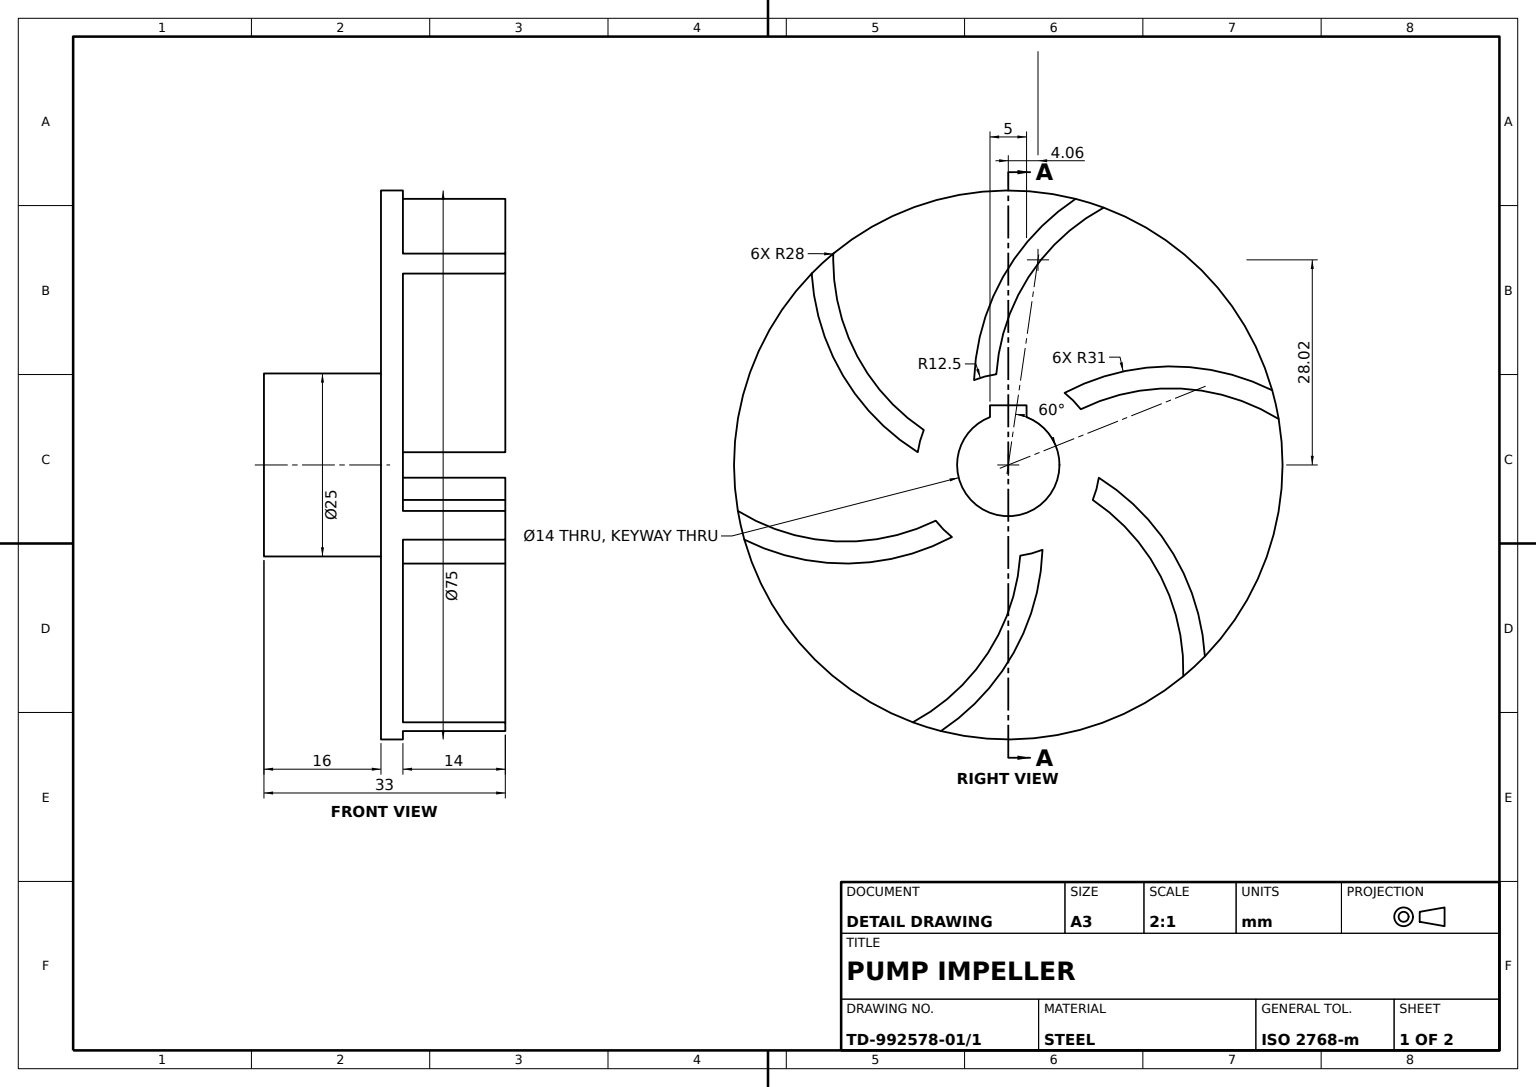
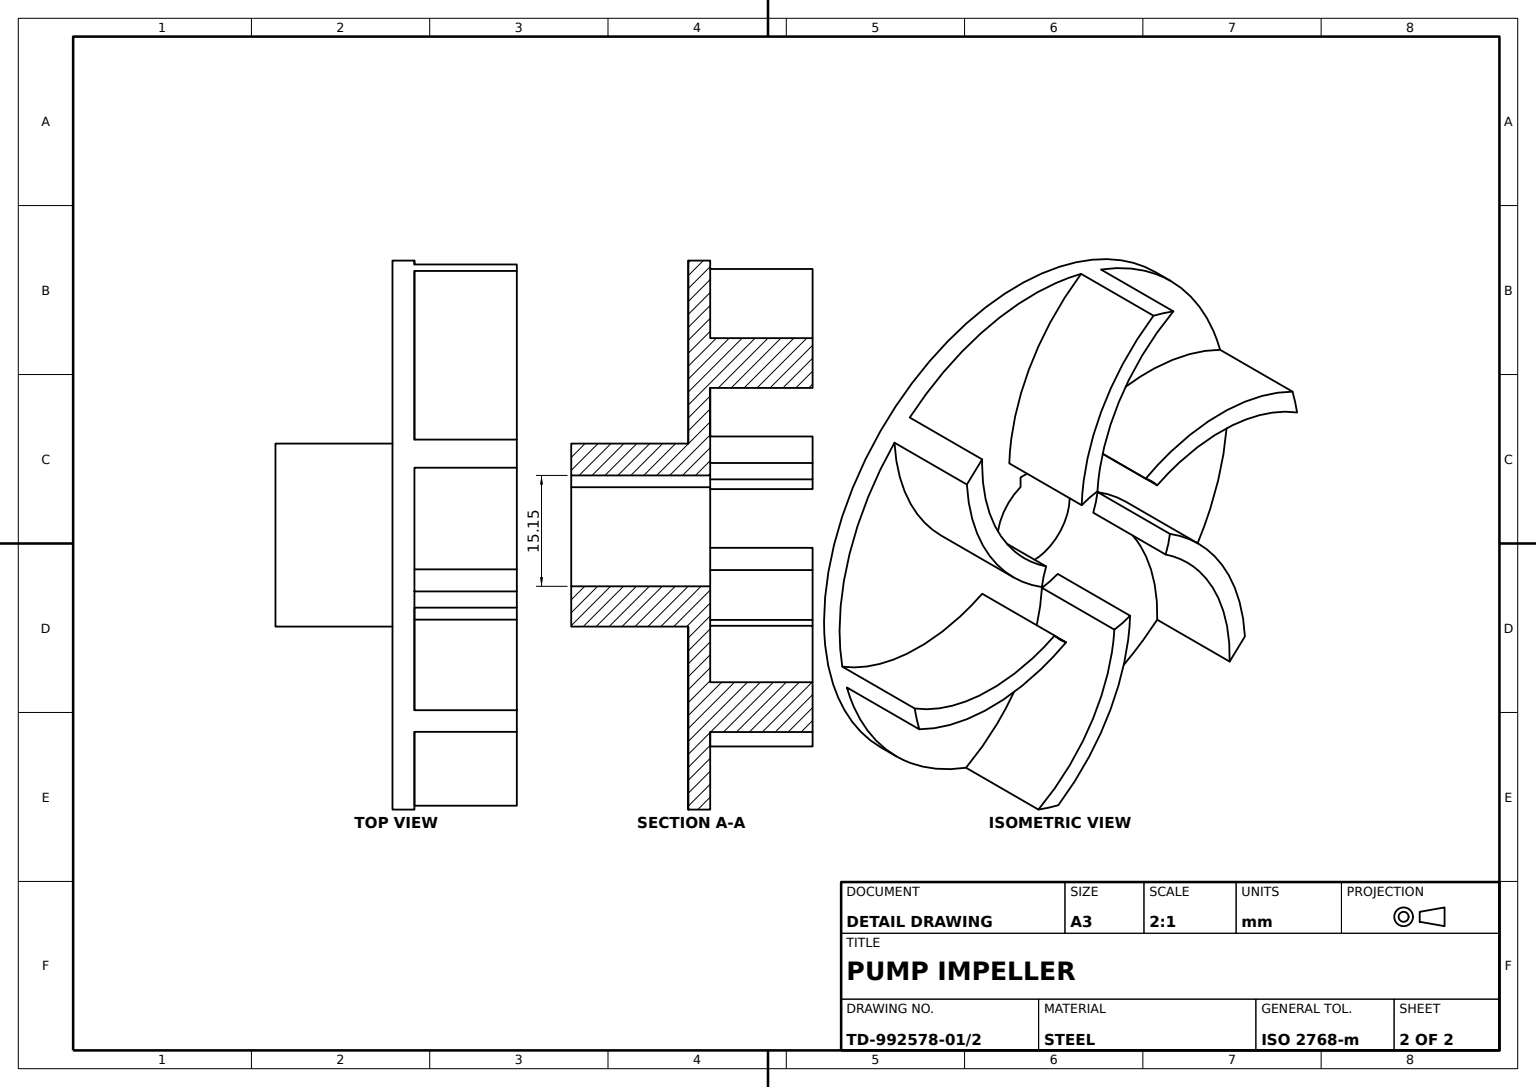
from build123d import *

# Parameters (mm, degrees)
SHAFT_BORE_PROFILE_W = 5
SHAFT_BORE_PROFILE_H = 2.3
SHAFT_BORE_DEPTH     = 30
VANES_6X_DEPTH       = 14


with BuildPart() as part:
    # Hub Disc Profile → Hub and Back Disc (revolve)
    with BuildSketch(Plane.XY, mode=Mode.PRIVATE) as hub_and_back_disc_sk:
        Polygon((0, 12.5), (0, 7), (19, 7), (19, 37.5), (16, 37.5), (16, 12.5), align=None)
    revolve(hub_and_back_disc_sk.sketch.rotate(Axis((-28, 0, 0), (1, 0, 0)), 90), axis=Axis((-28, 0, 0), (1, 0, 0)))

    # Shaft Bore Profile → Shaft Bore (cut)
    with BuildSketch(Plane.ZY):
        with Locations((0, 7)):
            Rectangle(SHAFT_BORE_PROFILE_W, SHAFT_BORE_PROFILE_H)
    extrude(amount=-SHAFT_BORE_DEPTH, mode=Mode.SUBTRACT)

    # Vane Profiles 6x → Vanes 6x (add)
    with BuildSketch(Plane(origin=(19, 0, 0), x_dir=(0, 0, -1), z_dir=(1, 0, 0))):
        with BuildLine():
            ThreePointArc((-36.970311015, -6.2806133), (-36.580104109, -8.255058047), (-36.084528464, -10.205724156))
            ThreePointArc((-36.084528464, -10.205724156), (-21.847293577, -13.468460533), (-7.696370779, -9.849663793))
            ThreePointArc((-7.696370779, -9.849663793), (-8.875739318, -8.801775478), (-9.913722012, -7.613679523))
            ThreePointArc((-9.913722012, -7.613679523), (-23.613958858, -10.436975539), (-36.970311015, -6.2806133))
        make_face()
        with BuildLine():
            ThreePointArc((-13.045984839, -35.157535175), (-11.140962076, -35.806828455), (-9.203847848, -36.352980411))
            ThreePointArc((-9.203847848, -36.352980411), (0.740382183, -25.654541508), (4.681873674, -11.590084508))
            ThreePointArc((4.681873674, -11.590084508), (3.184691504, -12.087503465), (1.636778877, -12.39237487))
            ThreePointArc((1.636778877, -12.39237487), (-2.768293473, -25.668776024), (-13.045984839, -35.157535175))
        make_face()
        with BuildLine():
            ThreePointArc((23.924326177, -28.876921875), (25.439142033, -27.551770408), (26.880680615, -26.147256255))
            ThreePointArc((26.880680615, -26.147256255), (22.58767576, -12.186080975), (12.378244453, -1.740420715))
            ThreePointArc((12.378244453, -1.740420715), (12.060430821, -3.285727987), (11.550500889, -4.778695347))
            ThreePointArc((11.550500889, -4.778695347), (20.845665384, -15.231800485), (23.924326177, -28.876921875))
        make_face()
        with BuildLine():
            ThreePointArc((-1.636778877, 12.39237487), (2.768293473, 25.668776024), (13.045984839, 35.157535175))
            ThreePointArc((13.045984839, 35.157535175), (11.140962076, 35.806828455), (9.203847848, 36.352980411))
            ThreePointArc((9.203847848, 36.352980411), (-0.740382183, 25.654541508), (-4.681873674, 11.590084508))
            ThreePointArc((-4.681873674, 11.590084508), (-3.184691504, 12.087503465), (-1.636778877, 12.39237487))
        make_face()
        with BuildLine():
            ThreePointArc((-23.924326177, 28.876921875), (-20.845665384, 15.231800485), (-11.550500889, 4.778695347))
            ThreePointArc((-11.550500889, 4.778695347), (-12.060430821, 3.285727987), (-12.378244453, 1.740420715))
            ThreePointArc((-12.378244453, 1.740420715), (-22.58767576, 12.186080975), (-26.880680615, 26.147256255))
            ThreePointArc((-26.880680615, 26.147256255), (-25.439142033, 27.551770408), (-23.924326177, 28.876921875))
        make_face()
        with BuildLine():
            ThreePointArc((36.084528464, 10.205724156), (21.847293577, 13.468460533), (7.696370779, 9.849663793))
            ThreePointArc((7.696370779, 9.849663793), (8.875739318, 8.801775478), (9.913722012, 7.613679523))
            ThreePointArc((9.913722012, 7.613679523), (23.613958858, 10.436975539), (36.970311015, 6.2806133))
            ThreePointArc((36.970311015, 6.2806133), (36.580104109, 8.255058047), (36.084528464, 10.205724156))
        make_face()
    extrude(amount=VANES_6X_DEPTH)


solid = part.part
